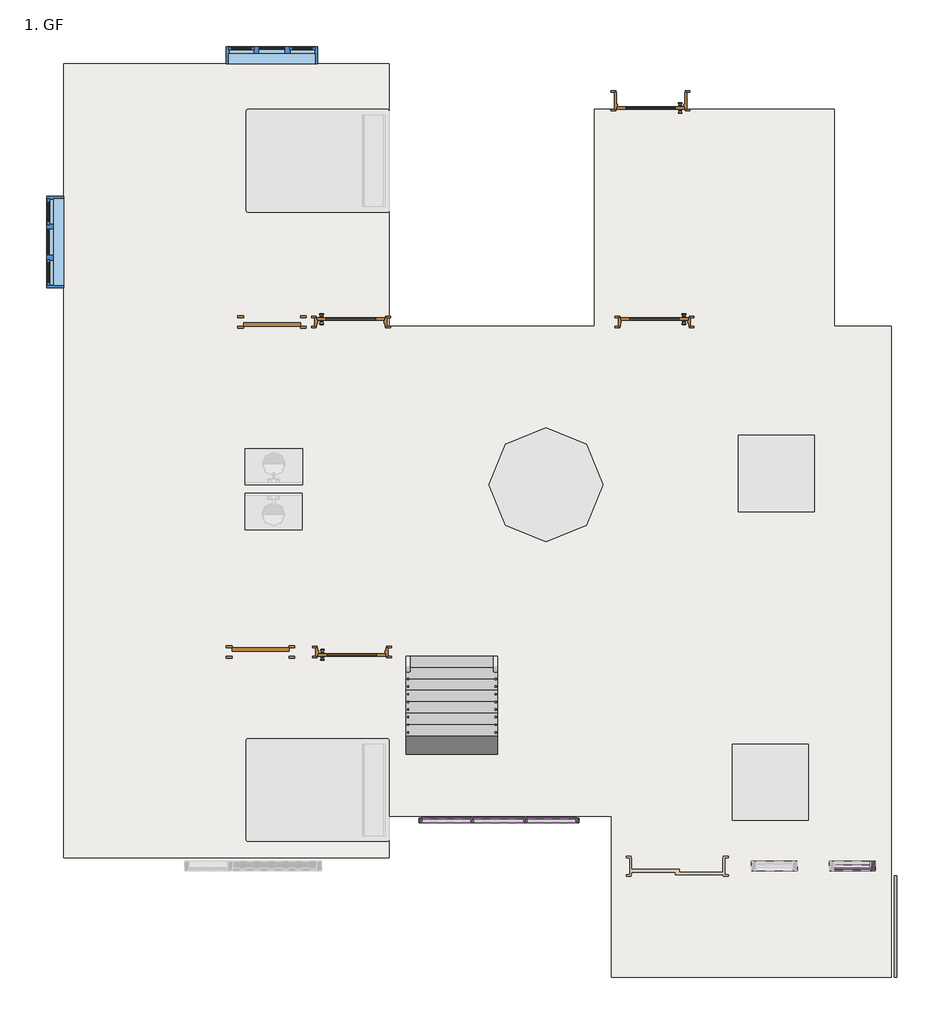
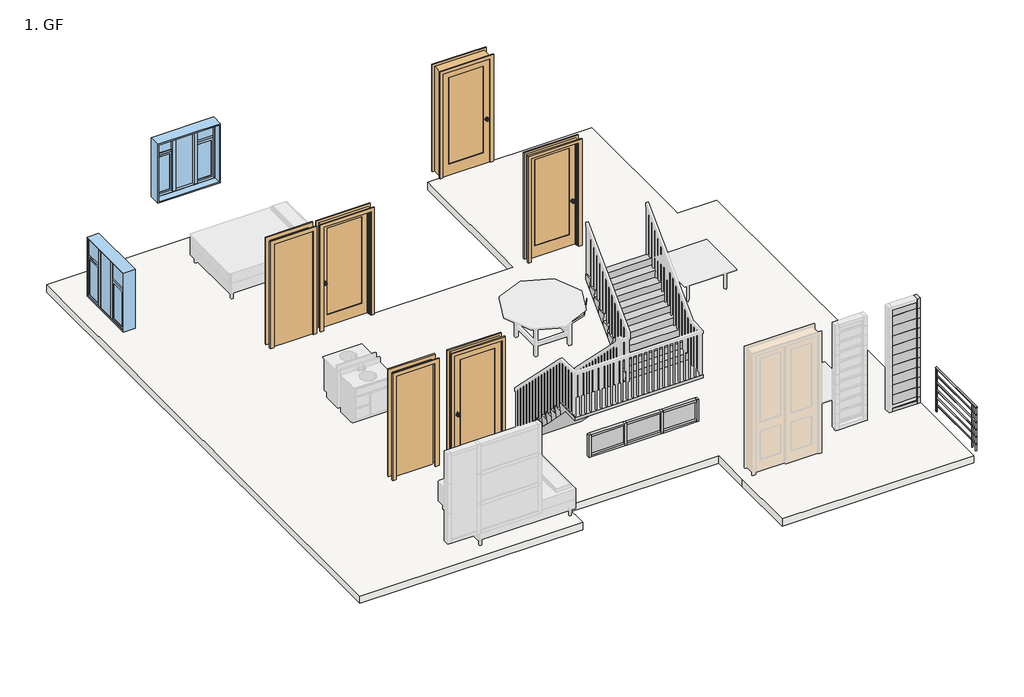
# One storey, part 2 of 3: 22 members, 13 plates, 6 doors, 2 windows, 1 railing, 1 slab, 1 stair flight.
"""IFC4 building model written with IfcOpenShell, lengths in millimetres."""

from ifc_helpers import new_model, si_unit, point, frame, frame_2d, origin, place, context, project, spatial, polyline, circle_curve, trimmed, segment, composite_curve, outline, extrude, faceted_brep, transform, mapped, element, save
from components import door_interior_single_1_panel_wood_4_x7_a3feeac7, door_interior_single_1_panel_wood_4_x7_3c6ab76a, door_interior_single_1_panel_wood_4_x7_3b97b8e7, door_214872d5, door_78caadf7, member_92f0adee, member_bf4473fa, member_7f78ed44, member_f6fe811f, member_86d06fe4, member_a8054089, member_a8e3eee7, system_panel_glazed_9eb8e914, system_panel_glazed_008e37cc, system_panel_glazed_f5251298, system_panel_glazed_d62326f9, window_casement_triple_side_transom_4_x4_fd24aed3

model = new_model("IFC4")

# Units and contexts
model_context = context("Model", 3, world=origin())
ifc_project = project(units=[si_unit("LENGTHUNIT", "METRE", prefix="MILLI")], contexts=[model_context])

# Site, building, storey
site = spatial("IfcSite", under=ifc_project)
building = spatial("IfcBuilding", under=site)
storey = spatial("IfcBuildingStorey", under=building, Name="1. GF", Elevation=609.6)

# Doors
placement = place(None, origin())
door_interior_single_1_panel_wood_4_x7_shape = door_interior_single_1_panel_wood_4_x7_a3feeac7(model_context)
element("IfcDoor", 1, ObjectType="Door-Interior-Single-1_Panel-Wood : 4'X7'", at=placement, inside=storey, context=model_context, shape_type="MappedRepresentation", body=[
    mapped(door_interior_single_1_panel_wood_4_x7_shape, transform((-3488.3749552, 2247.2410289, 609.6), x_axis=(1.0, 0.0, 0.0), y_axis=(0.0, 1.0, 0.0), z_axis=(0.0, 0.0, 1.0))),
])
element("IfcDoor", 2, ObjectType="Door-Interior-Single-1_Panel-Wood : 4'X7'", at=placement, inside=storey, context=model_context, shape_type="MappedRepresentation", body=[
    mapped(door_interior_single_1_panel_wood_4_x7_shape, transform((550.2250448, 6654.1410289, 609.6), x_axis=(-1.0, 0.0, 0.0), y_axis=(0.0, -1.0, 0.0), z_axis=(0.0, 0.0, 1.0))),
])
door_interior_single_1_panel_wood_4_x7_2_shape = door_interior_single_1_panel_wood_4_x7_3c6ab76a(model_context)
element("IfcDoor", 3, ObjectType="Door-Interior-Single-1_Panel-Wood : 4'X7'", at=placement, inside=storey, context=model_context, shape_type="MappedRepresentation", body=[
    mapped(door_interior_single_1_panel_wood_4_x7_2_shape, transform((-3501.0749552, 6654.1410289, 609.6), x_axis=(1.0, 0.0, 0.0), y_axis=(0.0, 1.0, 0.0), z_axis=(0.0, 0.0, 1.0))),
])
door_interior_single_1_panel_wood_4_x7_3_shape = door_interior_single_1_panel_wood_4_x7_3b97b8e7(model_context)
element("IfcDoor", 4, ObjectType="Door-Interior-Single-1_Panel-Wood : 4'X7'", at=placement, inside=storey, context=model_context, shape_type="MappedRepresentation", body=[
    mapped(door_interior_single_1_panel_wood_4_x7_3_shape, transform((499.4250448, 9600.5410289, 609.6), x_axis=(-1.0, 0.0, 0.0), y_axis=(0.0, -1.0, 0.0), z_axis=(0.0, 0.0, 1.0))),
])
door_shape = door_214872d5(model_context)
element("IfcDoor", 5, ObjectType="Single-Flush : 2'6\" X 7'", at=placement, inside=storey, context=model_context, shape_type="MappedRepresentation", body=[
    mapped(door_shape, transform((-4707.5749552, 2250.4160289, 609.6), x_axis=(1.0, 0.0, 0.0), y_axis=(0.0, 1.0, 0.0), z_axis=(0.0, 0.0, 1.0))),
])
door_2_shape = door_78caadf7(model_context)
element("IfcDoor", 6, ObjectType="Single-Flush : 2'6\" X 7'", at=placement, inside=storey, context=model_context, shape_type="MappedRepresentation", body=[
    mapped(door_2_shape, transform((-4555.1749552, 6650.9660289, 609.6), x_axis=(1.0, 0.0, 0.0), y_axis=(0.0, 1.0, 0.0), z_axis=(0.0, 0.0, 1.0))),
])

# Members
member_shape = member_92f0adee(model_context)
element("IfcMember", 7, ObjectType="Rectangular Mullion : 1.5\" x 2.5\" rectangular", at=placement, inside=storey, context=model_context, shape_type="MappedRepresentation", body=[
    mapped(member_shape, transform((-497.5249552, 2.5160289, 1981.2), x_axis=(0.0, 0.0, 1.0), y_axis=(0.0, -1.0, 0.0), z_axis=(1.0, 0.0, 0.0))),
])
element("IfcMember", 8, ObjectType="Rectangular Mullion : 1.5\" x 2.5\" rectangular", at=placement, inside=storey, context=model_context, shape_type="MappedRepresentation", body=[
    mapped(member_shape, transform((-1900.8749552, 2.5160289, 1981.2), x_axis=(0.0, 0.0, 1.0), y_axis=(0.0, -1.0, 0.0), z_axis=(1.0, 0.0, 0.0))),
])
element("IfcMember", 9, ObjectType="Rectangular Mullion : 1.5\" x 2.5\" rectangular", at=placement, inside=storey, context=model_context, shape_type="MappedRepresentation", body=[
    mapped(member_shape, transform((-2554.9249552, 2.5160289, 1524.0), x_axis=(0.0, 0.0, -1.0), y_axis=(0.0, -1.0, 0.0), z_axis=(-1.0, 0.0, 0.0))),
])
element("IfcMember", 10, ObjectType="Rectangular Mullion : 1.5\" x 2.5\" rectangular", at=placement, inside=storey, context=model_context, shape_type="MappedRepresentation", body=[
    mapped(member_shape, transform((-1151.5749552, 2.5160289, 1524.0), x_axis=(0.0, 0.0, -1.0), y_axis=(0.0, -1.0, 0.0), z_axis=(-1.0, 0.0, 0.0))),
])
member_2_shape = member_bf4473fa(model_context)
element("IfcMember", 11, ObjectType="Rectangular Mullion : 1.5\" x 2.5\" rectangular", at=placement, inside=storey, context=model_context, shape_type="MappedRepresentation", body=[
    mapped(member_2_shape, transform((-1881.8249552, 2.5160289, 1524.0), x_axis=(1.0, 0.0, 0.0), y_axis=(0.0, -1.0, 0.0), z_axis=(0.0, 0.0, -1.0))),
])
element("IfcMember", 12, ObjectType="Rectangular Mullion : 1.5\" x 2.5\" rectangular", at=placement, inside=storey, context=model_context, shape_type="MappedRepresentation", body=[
    mapped(member_2_shape, transform((-1170.6249552, 2.5160289, 1524.0), x_axis=(1.0, 0.0, 0.0), y_axis=(0.0, -1.0, 0.0), z_axis=(0.0, 0.0, -1.0))),
])
member_3_shape = member_7f78ed44(model_context)
element("IfcMember", 13, ObjectType="Rectangular Mullion : 1.5\" x 2.5\" rectangular", at=placement, inside=storey, context=model_context, shape_type="MappedRepresentation", body=[
    mapped(member_3_shape, transform((-1862.7749552, 2.5160289, 1524.0), x_axis=(0.0, 0.0, -1.0), y_axis=(0.0, -1.0, 0.0), z_axis=(-1.0, 0.0, 0.0))),
])
element("IfcMember", 14, ObjectType="Rectangular Mullion : 1.5\" x 2.5\" rectangular", at=placement, inside=storey, context=model_context, shape_type="MappedRepresentation", body=[
    mapped(member_3_shape, transform((-1189.6749552, 2.5160289, 1981.2), x_axis=(0.0, 0.0, 1.0), y_axis=(0.0, -1.0, 0.0), z_axis=(1.0, 0.0, 0.0))),
])
member_4_shape = member_f6fe811f(model_context)
element("IfcMember", 15, ObjectType="Rectangular Mullion : 1.5\" x 2.5\" rectangular", at=placement, inside=storey, context=model_context, shape_type="MappedRepresentation", body=[
    mapped(member_4_shape, transform((-2593.0249552, 2.5160289, 1981.2), x_axis=(-1.0, 0.0, 0.0), y_axis=(0.0, -1.0, 0.0), z_axis=(0.0, 0.0, 1.0))),
])
element("IfcMember", 16, ObjectType="Rectangular Mullion : 1.5\" x 2.5\" rectangular", at=placement, inside=storey, context=model_context, shape_type="MappedRepresentation", body=[
    mapped(member_4_shape, transform((-459.4249552, 2.5160289, 1524.0), x_axis=(1.0, 0.0, 0.0), y_axis=(0.0, -1.0, 0.0), z_axis=(0.0, 0.0, -1.0))),
])
member_5_shape = member_86d06fe4(model_context)
element("IfcMember", 17, ObjectType="Rectangular Mullion : 2.5\" x 5\" rectangular", at=placement, inside=storey, context=model_context, shape_type="MappedRepresentation", body=[
    mapped(member_5_shape, transform((3433.1250448, -607.0839711, 914.4), x_axis=(0.0, 0.0, -1.0), y_axis=(0.0, 1.0, 0.0), z_axis=(1.0, 0.0, 0.0))),
])
member_6_shape = member_a8054089(model_context)
element("IfcMember", 18, ObjectType="Rectangular Mullion : 2.5\" x 5\" rectangular", at=placement, inside=storey, context=model_context, shape_type="MappedRepresentation", body=[
    mapped(member_6_shape, transform((3496.6250448, -607.0839711, 3073.4), x_axis=(1.0, 0.0, 0.0), y_axis=(0.0, 1.0, 0.0), z_axis=(0.0, 0.0, 1.0))),
])
element("IfcMember", 19, ObjectType="Rectangular Mullion : 2.5\" x 5\" rectangular", at=placement, inside=storey, context=model_context, shape_type="MappedRepresentation", body=[
    mapped(member_6_shape, transform((3496.6250448, -607.0839711, 2870.2), x_axis=(1.0, 0.0, 0.0), y_axis=(0.0, 1.0, 0.0), z_axis=(0.0, 0.0, 1.0))),
])
element("IfcMember", 20, ObjectType="Rectangular Mullion : 2.5\" x 5\" rectangular", at=placement, inside=storey, context=model_context, shape_type="MappedRepresentation", body=[
    mapped(member_6_shape, transform((3496.6250448, -607.0839711, 2667.0), x_axis=(1.0, 0.0, 0.0), y_axis=(0.0, 1.0, 0.0), z_axis=(0.0, 0.0, 1.0))),
])
element("IfcMember", 21, ObjectType="Rectangular Mullion : 2.5\" x 5\" rectangular", at=placement, inside=storey, context=model_context, shape_type="MappedRepresentation", body=[
    mapped(member_6_shape, transform((3496.6250448, -607.0839711, 2463.8), x_axis=(1.0, 0.0, 0.0), y_axis=(0.0, 1.0, 0.0), z_axis=(0.0, 0.0, 1.0))),
])
element("IfcMember", 22, ObjectType="Rectangular Mullion : 2.5\" x 5\" rectangular", at=placement, inside=storey, context=model_context, shape_type="MappedRepresentation", body=[
    mapped(member_6_shape, transform((3496.6250448, -607.0839711, 2260.6), x_axis=(1.0, 0.0, 0.0), y_axis=(0.0, 1.0, 0.0), z_axis=(0.0, 0.0, 1.0))),
])
element("IfcMember", 23, ObjectType="Rectangular Mullion : 2.5\" x 5\" rectangular", at=placement, inside=storey, context=model_context, shape_type="MappedRepresentation", body=[
    mapped(member_6_shape, transform((3496.6250448, -607.0839711, 2057.4), x_axis=(1.0, 0.0, 0.0), y_axis=(0.0, 1.0, 0.0), z_axis=(0.0, 0.0, 1.0))),
])
element("IfcMember", 24, ObjectType="Rectangular Mullion : 2.5\" x 5\" rectangular", at=placement, inside=storey, context=model_context, shape_type="MappedRepresentation", body=[
    mapped(member_6_shape, transform((3496.6250448, -607.0839711, 1854.2), x_axis=(1.0, 0.0, 0.0), y_axis=(0.0, 1.0, 0.0), z_axis=(0.0, 0.0, 1.0))),
])
element("IfcMember", 25, ObjectType="Rectangular Mullion : 2.5\" x 5\" rectangular", at=placement, inside=storey, context=model_context, shape_type="MappedRepresentation", body=[
    mapped(member_6_shape, transform((3496.6250448, -607.0839711, 1651.0), x_axis=(1.0, 0.0, 0.0), y_axis=(0.0, 1.0, 0.0), z_axis=(0.0, 0.0, 1.0))),
])
element("IfcMember", 26, ObjectType="Rectangular Mullion : 2.5\" x 5\" rectangular", at=placement, inside=storey, context=model_context, shape_type="MappedRepresentation", body=[
    mapped(member_6_shape, transform((3496.6250448, -607.0839711, 1447.8), x_axis=(1.0, 0.0, 0.0), y_axis=(0.0, 1.0, 0.0), z_axis=(0.0, 0.0, 1.0))),
])
element("IfcMember", 27, ObjectType="Rectangular Mullion : 2.5\" x 5\" rectangular", at=placement, inside=storey, context=model_context, shape_type="MappedRepresentation", body=[
    mapped(member_6_shape, transform((3496.6250448, -607.0839711, 1244.6), x_axis=(1.0, 0.0, 0.0), y_axis=(0.0, 1.0, 0.0), z_axis=(0.0, 0.0, 1.0))),
])
member_7_shape = member_a8e3eee7(model_context)
element("IfcMember", 28, ObjectType="Rectangular Mullion : 2.5\" x 5\" rectangular", at=placement, inside=storey, context=model_context, shape_type="MappedRepresentation", body=[
    mapped(member_7_shape, transform((3496.6250448, -607.0839711, 1041.4), x_axis=(1.0, 0.0, 0.0), y_axis=(0.0, 1.0, 0.0), z_axis=(0.0, 0.0, 1.0))),
])

# Plates
system_panel_glazed_shape = system_panel_glazed_9eb8e914(model_context)
element("IfcPlate", 29, ObjectType="System Panel : Glazed", at=placement, inside=storey, context=model_context, shape_type="MappedRepresentation", body=[
    mapped(system_panel_glazed_shape, transform((3191.8250448, -607.0839711, 2667.0), x_axis=(-1.0, 0.0, 0.0), y_axis=(0.0, -1.0, 0.0), z_axis=(0.0, 0.0, 1.0))),
])
element("IfcPlate", 30, ObjectType="System Panel : Glazed", at=placement, inside=storey, context=model_context, shape_type="MappedRepresentation", body=[
    mapped(system_panel_glazed_shape, transform((3191.8250448, -607.0839711, 2463.8), x_axis=(-1.0, 0.0, 0.0), y_axis=(0.0, -1.0, 0.0), z_axis=(0.0, 0.0, 1.0))),
])
element("IfcPlate", 31, ObjectType="System Panel : Glazed", at=placement, inside=storey, context=model_context, shape_type="MappedRepresentation", body=[
    mapped(system_panel_glazed_shape, transform((3191.8250448, -607.0839711, 2260.6), x_axis=(-1.0, 0.0, 0.0), y_axis=(0.0, -1.0, 0.0), z_axis=(0.0, 0.0, 1.0))),
])
element("IfcPlate", 32, ObjectType="System Panel : Glazed", at=placement, inside=storey, context=model_context, shape_type="MappedRepresentation", body=[
    mapped(system_panel_glazed_shape, transform((3191.8250448, -607.0839711, 2057.4), x_axis=(-1.0, 0.0, 0.0), y_axis=(0.0, -1.0, 0.0), z_axis=(0.0, 0.0, 1.0))),
])
element("IfcPlate", 33, ObjectType="System Panel : Glazed", at=placement, inside=storey, context=model_context, shape_type="MappedRepresentation", body=[
    mapped(system_panel_glazed_shape, transform((3191.8250448, -607.0839711, 1854.2), x_axis=(-1.0, 0.0, 0.0), y_axis=(0.0, -1.0, 0.0), z_axis=(0.0, 0.0, 1.0))),
])
element("IfcPlate", 34, ObjectType="System Panel : Glazed", at=placement, inside=storey, context=model_context, shape_type="MappedRepresentation", body=[
    mapped(system_panel_glazed_shape, transform((3191.8250448, -607.0839711, 1651.0), x_axis=(-1.0, 0.0, 0.0), y_axis=(0.0, -1.0, 0.0), z_axis=(0.0, 0.0, 1.0))),
])
element("IfcPlate", 35, ObjectType="System Panel : Glazed", at=placement, inside=storey, context=model_context, shape_type="MappedRepresentation", body=[
    mapped(system_panel_glazed_shape, transform((3191.8250448, -607.0839711, 1447.8), x_axis=(-1.0, 0.0, 0.0), y_axis=(0.0, -1.0, 0.0), z_axis=(0.0, 0.0, 1.0))),
])
element("IfcPlate", 36, ObjectType="System Panel : Glazed", at=placement, inside=storey, context=model_context, shape_type="MappedRepresentation", body=[
    mapped(system_panel_glazed_shape, transform((3191.8250448, -607.0839711, 1244.6), x_axis=(-1.0, 0.0, 0.0), y_axis=(0.0, -1.0, 0.0), z_axis=(0.0, 0.0, 1.0))),
])
element("IfcPlate", 37, ObjectType="System Panel : Glazed", at=placement, inside=storey, context=model_context, shape_type="MappedRepresentation", body=[
    mapped(system_panel_glazed_shape, transform((3191.8250448, -607.0839711, 1041.4), x_axis=(-1.0, 0.0, 0.0), y_axis=(0.0, -1.0, 0.0), z_axis=(0.0, 0.0, 1.0))),
])
system_panel_glazed_2_shape = system_panel_glazed_008e37cc(model_context)
element("IfcPlate", 38, ObjectType="System Panel : Glazed", at=placement, inside=storey, context=model_context, shape_type="MappedRepresentation", body=[
    mapped(system_panel_glazed_2_shape, transform((3191.8250448, -607.0839711, 2870.2), x_axis=(-1.0, 0.0, 0.0), y_axis=(0.0, -1.0, 0.0), z_axis=(0.0, 0.0, 1.0))),
])
system_panel_glazed_3_shape = system_panel_glazed_f5251298(model_context)
element("IfcPlate", 39, ObjectType="System Panel : Glazed", at=placement, inside=storey, context=model_context, shape_type="MappedRepresentation", body=[
    mapped(system_panel_glazed_3_shape, transform((-2227.8999552, 2.5160289, 1562.1), x_axis=(1.0, 0.0, 0.0), y_axis=(0.0, 1.0, 0.0), z_axis=(0.0, 0.0, 1.0))),
])
element("IfcPlate", 40, ObjectType="System Panel : Glazed", at=placement, inside=storey, context=model_context, shape_type="MappedRepresentation", body=[
    mapped(system_panel_glazed_3_shape, transform((-824.5499552, 2.5160289, 1562.1), x_axis=(1.0, 0.0, 0.0), y_axis=(0.0, 1.0, 0.0), z_axis=(0.0, 0.0, 1.0))),
])
system_panel_glazed_4_shape = system_panel_glazed_d62326f9(model_context)
element("IfcPlate", 41, ObjectType="System Panel : Glazed", at=placement, inside=storey, context=model_context, shape_type="MappedRepresentation", body=[
    mapped(system_panel_glazed_4_shape, transform((-1526.2249552, 2.5160289, 1562.1), x_axis=(1.0, 0.0, 0.0), y_axis=(0.0, 1.0, 0.0), z_axis=(0.0, 0.0, 1.0))),
])

# Railing
element("IfcRailing", 42, ObjectType="Handrail - Pipe", at=placement, inside=storey, context=model_context, shape_type="SweptSolid", body=[
    extrude(outline(composite_curve([segment(trimmed(circle_curve(frame_2d((1579.959375, 3769.6750448)), 19.05), [point((1579.959375, 3750.6250448))], [point((1579.959375, 3788.7250448))], False, "CARTESIAN"), True, "CONTINUOUS"), segment(trimmed(circle_curve(frame_2d((1579.959375, 3769.6750448)), 19.05), [point((1579.959375, 3788.7250448))], [point((1579.959375, 3750.6250448))], False, "CARTESIAN"), True, "CONTINUOUS")], self_intersect=False)), frame((0.0, -2092.7839711, 0.0), z_axis=(0.0, 1.0, 0.0), x_axis=(0.0, 0.0, 1.0)), (0.0, 0.0, 1.0), 1358.7),
    extrude(outline(composite_curve([segment(trimmed(circle_curve(frame_2d((1433.909375, 3769.6750448)), 12.7), [point((1433.909375, 3782.3750448))], [point((1433.909375, 3756.9750448))], False, "CARTESIAN"), True, "CONTINUOUS"), segment(trimmed(circle_curve(frame_2d((1433.909375, 3769.6750448)), 12.7), [point((1433.909375, 3756.9750448))], [point((1433.909375, 3782.3750448))], False, "CARTESIAN"), True, "CONTINUOUS")], self_intersect=False)), frame((0.0, -2092.7839711, 0.0), z_axis=(0.0, 1.0, 0.0), x_axis=(0.0, 0.0, 1.0)), (0.0, 0.0, 1.0), 1358.7),
    extrude(outline(composite_curve([segment(trimmed(circle_curve(frame_2d((1281.509375, 3769.6750448)), 12.7), [point((1281.509375, 3782.3750448))], [point((1281.509375, 3756.9750448))], False, "CARTESIAN"), True, "CONTINUOUS"), segment(trimmed(circle_curve(frame_2d((1281.509375, 3769.6750448)), 12.7), [point((1281.509375, 3756.9750448))], [point((1281.509375, 3782.3750448))], False, "CARTESIAN"), True, "CONTINUOUS")], self_intersect=False)), frame((0.0, -2092.7839711, 0.0), z_axis=(0.0, 1.0, 0.0), x_axis=(0.0, 0.0, 1.0)), (0.0, 0.0, 1.0), 1358.7),
    extrude(outline(composite_curve([segment(trimmed(circle_curve(frame_2d((1129.109375, 3769.6750448)), 12.7), [point((1129.109375, 3782.3750448))], [point((1129.109375, 3756.9750448))], False, "CARTESIAN"), True, "CONTINUOUS"), segment(trimmed(circle_curve(frame_2d((1129.109375, 3769.6750448)), 12.7), [point((1129.109375, 3756.9750448))], [point((1129.109375, 3782.3750448))], False, "CARTESIAN"), True, "CONTINUOUS")], self_intersect=False)), frame((0.0, -2092.7839711, 0.0), z_axis=(0.0, 1.0, 0.0), x_axis=(0.0, 0.0, 1.0)), (0.0, 0.0, 1.0), 1358.7),
    extrude(outline(composite_curve([segment(trimmed(circle_curve(frame_2d((976.709375, 3769.6750448)), 12.7), [point((976.709375, 3782.3750448))], [point((976.709375, 3756.9750448))], False, "CARTESIAN"), True, "CONTINUOUS"), segment(trimmed(circle_curve(frame_2d((976.709375, 3769.6750448)), 12.7), [point((976.709375, 3756.9750448))], [point((976.709375, 3782.3750448))], False, "CARTESIAN"), True, "CONTINUOUS")], self_intersect=False)), frame((0.0, -2092.7839711, 0.0), z_axis=(0.0, 1.0, 0.0), x_axis=(0.0, 0.0, 1.0)), (0.0, 0.0, 1.0), 1358.7),
    extrude(outline(composite_curve([segment(trimmed(circle_curve(frame_2d((824.309375, 3769.6750448)), 12.7), [point((824.309375, 3782.3750448))], [point((824.309375, 3756.9750448))], False, "CARTESIAN"), True, "CONTINUOUS"), segment(trimmed(circle_curve(frame_2d((824.309375, 3769.6750448)), 12.7), [point((824.309375, 3756.9750448))], [point((824.309375, 3782.3750448))], False, "CARTESIAN"), True, "CONTINUOUS")], self_intersect=False)), frame((0.0, -2092.7839711, 0.0), z_axis=(0.0, 1.0, 0.0), x_axis=(0.0, 0.0, 1.0)), (0.0, 0.0, 1.0), 1358.7),
    extrude(outline(composite_curve([segment(trimmed(circle_curve(frame_2d((3769.6750448, -1953.2839711)), 12.7), [point((3782.3750448, -1953.2839711))], [point((3756.9750448, -1953.2839711))], False, "CARTESIAN"), True, "CONTINUOUS"), segment(trimmed(circle_curve(frame_2d((3769.6750448, -1953.2839711)), 12.7), [point((3756.9750448, -1953.2839711))], [point((3782.3750448, -1953.2839711))], False, "CARTESIAN"), True, "CONTINUOUS")], self_intersect=False)), frame((0.0, 0.0, 684.609375), z_axis=(0.0, 0.0, 1.0), x_axis=(1.0, 0.0, 0.0)), (0.0, 0.0, 1.0), 876.3),
    extrude(outline(composite_curve([segment(trimmed(circle_curve(frame_2d((3769.6750448, -2080.0839711)), 12.7), [point((3782.3750448, -2080.0839711))], [point((3756.9750448, -2080.0839711))], False, "CARTESIAN"), True, "CONTINUOUS"), segment(trimmed(circle_curve(frame_2d((3769.6750448, -2080.0839711)), 12.7), [point((3756.9750448, -2080.0839711))], [point((3782.3750448, -2080.0839711))], False, "CARTESIAN"), True, "CONTINUOUS")], self_intersect=False)), frame((0.0, 0.0, 684.609375), z_axis=(0.0, 0.0, 1.0), x_axis=(1.0, 0.0, 0.0)), (0.0, 0.0, 1.0), 876.3),
    extrude(outline(composite_curve([segment(trimmed(circle_curve(frame_2d((3769.6750448, -746.7839711)), 12.7), [point((3782.3750448, -746.7839711))], [point((3756.9750448, -746.7839711))], False, "CARTESIAN"), True, "CONTINUOUS"), segment(trimmed(circle_curve(frame_2d((3769.6750448, -746.7839711)), 12.7), [point((3756.9750448, -746.7839711))], [point((3782.3750448, -746.7839711))], False, "CARTESIAN"), True, "CONTINUOUS")], self_intersect=False)), frame((0.0, 0.0, 684.609375), z_axis=(0.0, 0.0, 1.0), x_axis=(1.0, 0.0, 0.0)), (0.0, 0.0, 1.0), 876.3),
])

# Slab
element("IfcSlab", 43, ObjectType="6\" FLOOR", at=placement, inside=storey, context=model_context, shape_type="SweptSolid", body=[
    extrude(outline(polyline([(-2993.0749552, 10099.0160289), (-2993.0749552, 6593.8160289), (-249.8749552, 6593.8160289), (-249.8749552, 9489.4160289), (2950.5250448, 9489.4160289), (2950.5250448, 6708.1160289), (2950.5250448, 6593.8160289), (3712.5250448, 6593.8160289), (3712.5250448, -492.7839711), (3712.5250448, -2092.7839711), (-21.2749552, -2092.7839711), (-21.2749552, -728.4733894), (-21.2749552, 59.6660289), (-2993.0749552, 59.6660289), (-2993.0749552, -492.7839711), (-7336.4749552, -492.7839711), (-7336.4749552, 10099.0160289), (-2993.0749552, 10099.0160289)])), frame((0.0, 0.0, 457.2), z_axis=(0.0, 0.0, 1.0), x_axis=(1.0, 0.0, 0.0)), (0.0, 0.0, 1.0), 152.4),
])

# Stair flight
element("IfcStairFlight", 44, ObjectType="3/4\" Nosing", at=placement, inside=storey, context=model_context, shape_type="Brep", body=[
    faceted_brep([(-2764.4749552, 2193.2660289, 762.0), (-1545.2749552, 2193.2660289, 762.0), (-1545.2749552, 2174.2160289, 609.6), (-2764.4749552, 2174.2160289, 609.6), (-2764.4749552, 2021.8160289, 762.0), (-1545.2749552, 2021.8160289, 762.0), (-1545.2749552, 2021.8160289, 672.1974388), (-1545.2749552, 2084.4134676, 609.6), (-2764.4749552, 2084.4134676, 609.6), (-2764.4749552, 2021.8160289, 672.1974388), (-1545.2749552, 2040.8660289, 914.4), (-2764.4749552, 2040.8660289, 914.4), (-2764.4749552, 1869.4160289, 914.4), (-1545.2749552, 1869.4160289, 914.4), (-1545.2749552, 1869.4160289, 824.5974388), (-2764.4749552, 1869.4160289, 824.5974388), (-1545.2749552, 1888.4660289, 1066.8), (-2764.4749552, 1888.4660289, 1066.8), (-2764.4749552, 1717.0160289, 1066.8), (-1545.2749552, 1717.0160289, 1066.8), (-1545.2749552, 1717.0160289, 976.9974388), (-2764.4749552, 1717.0160289, 976.9974388), (-1545.2749552, 1736.0660289, 1219.2), (-2764.4749552, 1736.0660289, 1219.2), (-2764.4749552, 1564.6160289, 1219.2), (-1545.2749552, 1564.6160289, 1219.2), (-1545.2749552, 1564.6160289, 1129.3974388), (-2764.4749552, 1564.6160289, 1129.3974388), (-1545.2749552, 1583.6660289, 1371.6), (-2764.4749552, 1583.6660289, 1371.6), (-2764.4749552, 1412.2160289, 1371.6), (-1545.2749552, 1412.2160289, 1371.6), (-1545.2749552, 1412.2160289, 1281.7974388), (-2764.4749552, 1412.2160289, 1281.7974388), (-1545.2749552, 1431.2660289, 1524.0), (-2764.4749552, 1431.2660289, 1524.0), (-2764.4749552, 1259.8160289, 1524.0), (-1545.2749552, 1259.8160289, 1524.0), (-1545.2749552, 1259.8160289, 1434.1974388), (-2764.4749552, 1259.8160289, 1434.1974388), (-1545.2749552, 1278.8660289, 1676.4), (-2764.4749552, 1278.8660289, 1676.4), (-2764.4749552, 1107.4160289, 1676.4), (-1545.2749552, 1107.4160289, 1676.4), (-1545.2749552, 1107.4160289, 1586.5974388), (-2764.4749552, 1107.4160289, 1586.5974388), (-1545.2749552, 1126.4660289, 1828.8), (-2764.4749552, 1126.4660289, 1828.8), (-2764.4749552, 955.0160289, 1828.8), (-1545.2749552, 955.0160289, 1828.8), (-1545.2749552, 955.0160289, 1738.9974388), (-2764.4749552, 955.0160289, 1738.9974388), (-1545.2749552, 974.0660289, 1981.2), (-2764.4749552, 974.0660289, 1981.2), (-2764.4749552, 802.6160289, 1981.2), (-1545.2749552, 802.6160289, 1981.2), (-1545.2749552, 802.6160289, 1891.3974388), (-2764.4749552, 802.6160289, 1891.3974388), (-1545.2749552, 650.2160289, 2133.6), (-1545.2749552, 821.6660289, 2133.6), (-2764.4749552, 821.6660289, 2133.6), (-2764.4749552, 650.2160289, 2133.6), (-1545.2749552, 661.3285289, 2222.5), (-1545.2749552, 471.5134676, 2222.5), (-2764.4749552, 650.2160289, 2043.7974388), (-1469.0749552, 688.3160289, 2286.0), (-1469.0749552, 669.2660289, 2286.0), (-1545.2749552, 669.2660289, 2286.0), (-2764.4749552, 669.2660289, 2286.0), (-2764.4749552, 471.5134676, 2286.0), (-2764.4749552, 173.9660289, 2286.0), (-249.8749552, 173.9660289, 2286.0), (-249.8749552, 688.3160289, 2286.0), (-1469.0749552, 688.3160289, 2222.5), (-1469.0749552, 669.2660289, 2222.5), (-1545.2749552, 669.2660289, 2222.5), (-2764.4749552, 471.5134676, 2222.5), (-2764.4749552, 173.9660289, 2222.5), (-249.8749552, 173.9660289, 2222.5), (-249.8749552, 688.3160289, 2222.5), (-1469.0749552, 669.2660289, 2438.4), (-249.8749552, 669.2660289, 2438.4), (-249.8749552, 714.6185901, 2438.4), (-249.8749552, 840.7160289, 2438.4), (-1469.0749552, 840.7160289, 2438.4), (-1469.0749552, 714.6185901, 2438.4), (-1469.0749552, 840.7160289, 2348.5974388), (-1469.0749552, 714.6185901, 2222.5), (-249.8749552, 714.6185901, 2222.5), (-249.8749552, 840.7160289, 2348.5974388), (-1469.0749552, 821.6660289, 2590.8), (-249.8749552, 821.6660289, 2590.8), (-249.8749552, 993.1160289, 2590.8), (-1469.0749552, 993.1160289, 2590.8), (-1469.0749552, 993.1160289, 2500.9974388), (-249.8749552, 993.1160289, 2500.9974388), (-1469.0749552, 974.0660289, 2743.2), (-249.8749552, 974.0660289, 2743.2), (-249.8749552, 1145.5160289, 2743.2), (-1469.0749552, 1145.5160289, 2743.2), (-1469.0749552, 1145.5160289, 2653.3974388), (-249.8749552, 1145.5160289, 2653.3974388), (-1469.0749552, 1126.4660289, 2895.6), (-249.8749552, 1126.4660289, 2895.6), (-249.8749552, 1297.9160289, 2895.6), (-1469.0749552, 1297.9160289, 2895.6), (-1469.0749552, 1297.9160289, 2805.7974388), (-249.8749552, 1297.9160289, 2805.7974388), (-1469.0749552, 1278.8660289, 3048.0), (-249.8749552, 1278.8660289, 3048.0), (-249.8749552, 1450.3160289, 3048.0), (-1469.0749552, 1450.3160289, 3048.0), (-1469.0749552, 1450.3160289, 2958.1974388), (-249.8749552, 1450.3160289, 2958.1974388), (-1469.0749552, 1431.2660289, 3200.4), (-249.8749552, 1431.2660289, 3200.4), (-249.8749552, 1602.7160289, 3200.4), (-1469.0749552, 1602.7160289, 3200.4), (-1469.0749552, 1602.7160289, 3110.5974388), (-249.8749552, 1602.7160289, 3110.5974388), (-1469.0749552, 1583.6660289, 3352.8), (-249.8749552, 1583.6660289, 3352.8), (-249.8749552, 1755.1160289, 3352.8), (-1469.0749552, 1755.1160289, 3352.8), (-1469.0749552, 1755.1160289, 3262.9974388), (-249.8749552, 1755.1160289, 3262.9974388), (-1469.0749552, 1736.0660289, 3505.2), (-249.8749552, 1736.0660289, 3505.2), (-249.8749552, 1907.5160289, 3505.2), (-1469.0749552, 1907.5160289, 3505.2), (-1469.0749552, 1907.5160289, 3415.3974388), (-249.8749552, 1907.5160289, 3415.3974388), (-1469.0749552, 1888.4660289, 3657.6), (-249.8749552, 1888.4660289, 3657.6), (-249.8749552, 2040.8660289, 3657.6), (-1469.0749552, 2040.8660289, 3657.6), (-1469.0749552, 2040.8660289, 3548.7474388), (-249.8749552, 2040.8660289, 3548.7474388)], [[[0, 1, 2, 3]], [[1, 0, 4, 5]], [[1, 5, 6, 7, 2]], [[4, 0, 3, 8, 9]], [[10, 11, 12, 13]], [[10, 13, 14, 6, 5]], [[12, 11, 4, 9, 15]], [[5, 4, 11, 10]], [[16, 17, 18, 19]], [[16, 19, 20, 14, 13]], [[18, 17, 12, 15, 21]], [[13, 12, 17, 16]], [[22, 23, 24, 25]], [[22, 25, 26, 20, 19]], [[24, 23, 18, 21, 27]], [[19, 18, 23, 22]], [[28, 29, 30, 31]], [[28, 31, 32, 26, 25]], [[30, 29, 24, 27, 33]], [[25, 24, 29, 28]], [[34, 35, 36, 37]], [[34, 37, 38, 32, 31]], [[36, 35, 30, 33, 39]], [[31, 30, 35, 34]], [[40, 41, 42, 43]], [[40, 43, 44, 38, 37]], [[42, 41, 36, 39, 45]], [[37, 36, 41, 40]], [[46, 47, 48, 49]], [[46, 49, 50, 44, 43]], [[48, 47, 42, 45, 51]], [[43, 42, 47, 46]], [[52, 53, 54, 55]], [[52, 55, 56, 50, 49]], [[54, 53, 48, 51, 57]], [[49, 48, 53, 52]], [[58, 59, 60, 61]], [[58, 62, 63, 56, 55, 59]], [[61, 60, 54, 57, 64]], [[55, 54, 60, 59]], [[65, 66, 67, 68, 69, 70, 71, 72]], [[66, 65, 73, 74]], [[67, 66, 74, 75]], [[62, 67, 75]], [[68, 61, 64, 76, 77, 70, 69]], [[71, 70, 77, 78]], [[72, 71, 78, 79]], [[58, 61, 68, 67, 62]], [[80, 81, 82, 83, 84, 85]], [[65, 80, 85, 84, 86, 87, 73]], [[81, 72, 79, 88, 89, 83, 82]], [[65, 72, 81, 80]], [[90, 91, 92, 93]], [[90, 93, 94, 86, 84]], [[92, 91, 83, 89, 95]], [[84, 83, 91, 90]], [[96, 97, 98, 99]], [[96, 99, 100, 94, 93]], [[98, 97, 92, 95, 101]], [[93, 92, 97, 96]], [[102, 103, 104, 105]], [[102, 105, 106, 100, 99]], [[104, 103, 98, 101, 107]], [[99, 98, 103, 102]], [[108, 109, 110, 111]], [[108, 111, 112, 106, 105]], [[110, 109, 104, 107, 113]], [[105, 104, 109, 108]], [[114, 115, 116, 117]], [[114, 117, 118, 112, 111]], [[116, 115, 110, 113, 119]], [[111, 110, 115, 114]], [[120, 121, 122, 123]], [[120, 123, 124, 118, 117]], [[122, 121, 116, 119, 125]], [[117, 116, 121, 120]], [[126, 127, 128, 129]], [[126, 129, 130, 124, 123]], [[128, 127, 122, 125, 131]], [[123, 122, 127, 126]], [[132, 133, 134, 135]], [[132, 135, 136, 130, 129]], [[134, 133, 128, 131, 137]], [[135, 134, 137, 136]], [[129, 128, 133, 132]], [[3, 2, 7, 8]], [[56, 63, 76, 64, 57, 51, 45, 39, 33, 27, 21, 15, 9, 8, 7, 6, 14, 20, 26, 32, 38, 44, 50]], [[76, 63, 62, 75, 74, 73, 87, 88, 79, 78, 77]], [[88, 87, 86, 94, 100, 106, 112, 118, 124, 130, 136, 137, 131, 125, 119, 113, 107, 101, 95, 89]]]),
])

# Windows
window_casement_triple_side_transom_4_x4_shape = window_casement_triple_side_transom_4_x4_fd24aed3(model_context)
element("IfcWindow", 45, ObjectType="Window-Casement-Triple-Side-Transom : 4'x4'", at=placement, inside=storey, context=model_context, shape_type="MappedRepresentation", body=[
    mapped(window_casement_triple_side_transom_4_x4_shape, transform((-4555.1749552, 10213.3160289, 609.6), x_axis=(1.0, 0.0, 0.0), y_axis=(0.0, 1.0, 0.0), z_axis=(0.0, 0.0, 1.0))),
])
element("IfcWindow", 46, ObjectType="Window-Casement-Triple-Side-Transom : 4'x4'", at=placement, inside=storey, context=model_context, shape_type="MappedRepresentation", body=[
    mapped(window_casement_triple_side_transom_4_x4_shape, transform((-7450.7749552, 7717.7660289, 609.6), x_axis=(0.0, 1.0, 0.0), y_axis=(-1.0, 0.0, 0.0), z_axis=(0.0, 0.0, 1.0))),
])

save(model, "model.ifc")

# Revit data of these elements
# Type "Door-Interior-Single-1_Panel-Wood : 4'X7'"
#   Type Mark = "9"
#   Assembly Code = "C1020300"
#   Analytic Construction = "Wooden"
#   Top Rail = 0' - 4 11/16"
#   Thickness = 0' - 1 3/8"
#   Thermal Resistance (R) = 2.5876 (h·ft²·°F)/BTU
#   Swing Angle [instance default] = 90.00°
#   Stiles = 0' - 4 3/4"
#   Rough Width = 3' - 2"
#   Rough Height = 7' - 1"
#   Height = 7' - 0"
#   Width = 3' - 0"
#   Heat Transfer Coefficient (U) = 0.3865 BTU/(h·ft²·°F)
#   Bottom Rail = 0' - 9 1/8"
#   Trim Material = Cherry
#   Panel Material = Cherry
#   Frame Material = Cherry
#   Door Handle Material = Aluminum
#   Visual Light Transmittance = 0
#   Solar Heat Gain Coefficient = 0
#   Wall Closure = (empty or 0)
#   Function = (empty or 0)
# Type "Single-Flush : 2'6\" X 7'"
#   Type Mark = "14"
#   Construction Type Id = "MDOOR"
#   Assembly Code = "C1020"
#   Analytic Construction = "Metal"
#   Thickness = 0' - 2"
#   Heat Transfer Coefficient (U) = 0.651978 BTU/(h·ft²·°F)
#   Height = 7' - 0"
#   Trim Projection Ext = 0' - 1"
#   Trim Projection Int = 0' - 1"
#   Trim Width = 0' - 3"
#   Width = 2' - 6"
#   Define Thermal Properties by = 1
#   Door Material = Door - Panel
#   Frame Material = Door - Frame
#   Visual Light Transmittance = 0
#   Solar Heat Gain Coefficient = 0
#   Function = (empty or 0)
#   Wall Closure = (empty or 0)
# Type "Rectangular Mullion : 1.5\" x 2.5\" rectangular"
#   built-in parameter 1007304 = 0.208333 (stored number, unit not read)
#   built-in parameter 1007301 = 0.0625 (stored number, unit not read)
#   built-in parameter 1007300 = 0.0625 (stored number, unit not read)
# Type "Rectangular Mullion : 2.5\" x 5\" rectangular"
#   built-in parameter 1007304 = 0.416667 (stored number, unit not read)
#   built-in parameter 1007301 = 0.104167 (stored number, unit not read)
#   built-in parameter 1007300 = 0.104167 (stored number, unit not read)
# Type "System Panel : Glazed"
#   Construction Type Id = "GSP4R"
#   Analytic Construction = "1/8 in Pilkington single glazing"
#   Visual Light Transmittance = 0.9
#   Solar Heat Gain Coefficient = 0.86
#   Heat Transfer Coefficient (U) = 1.18115 BTU/(h·ft²·°F)
#   Define Thermal Properties by = 1
# Type "Handrail - Pipe"
#   Assembly Code = "C2010400"
#   built-in parameter 1008612 = 0.0416667 (stored number, unit not read)
#   built-in parameter 1008611 = 0.0833333 (stored number, unit not read)
#   built-in parameter 1008609 = 4 (stored number, unit not read)
#   built-in parameter 1008604 = 0.166667 (stored number, unit not read)
#   built-in parameter 1008603 = 0.166667 (stored number, unit not read)
#   Railing Height = 3' - 0"
#   built-in parameter 1008630 = 2
#   built-in parameter 1008610 = 1
#   built-in parameter 1008605 = 1
#   built-in parameter 1008618 = Baluster - Round : 1"
# Type "6\" FLOOR"
#   Assembly Code = "B1010"
#   Function = 0
#   Layers, outside or top first: 0' - 6" "Gypsum Wall Board" (function 1)
# Type "Window-Casement-Triple-Side-Transom : 4'x4'"
#   Type Mark = "27"
#   Fire Rating = "0.5h"
#   Assembly Code = "B2020100"
#   Analytic Construction = "Double glazing - domestic"
#   Window Width = 1' - 4"
#   Window Inset [instance default] = 0' - 0 5/8"
#   Wall Thickness [instance default] = 0' - 6"
#   Visual Light Transmittance = 0.81
#   Transom Height Ratio = 0.3
#   Thermal Resistance (R) = 1.8146 (h·ft²·°F)/BTU
#   Solar Heat Gain Coefficient = 0.76
#   Rough Width = 4' - 0 1/2"
#   Rough Height = 4' - 0 1/2"
#   Open Window Height = 2' - 9.6"
#   Heat Transfer Coefficient (U) = 0.5511 BTU/(h·ft²·°F)
#   Height = 4' - 0"
#   Transom Height = 1' - 2.4"
#   Frame Gap 3 [instance default] = 0' - 1 83/128"
#   Frame Gap 2 [instance default] = 0' - 0 5/8"
#   Frame Gap 1 = 0' - 1 51/128"
#   Default Sill Height = 3' - 0"
#   Width = 4' - 0"
#   Frame Material = Metal - Aluminum
#   Glass Panel Material = Glass
#   Wall Closure = (empty or 0)
# Elements 1, 2, 3, 4 (IfcDoor, "Door-Interior-Single-1_Panel-Wood : 4'X7'")
#   Swing Angle = 90.00°
#   Phase Created = New Construction
#   Materials on its faces: "Cherry", "Aluminum"
# Elements 5, 6 (IfcDoor, "Single-Flush : 2'6\" X 7'")
#   Phase Created = New Construction
#   Materials on its faces: "Door - Frame", "Door - Panel"
# Elements 7, 8, 9, 10, 11, 12, 13, 14, 15, 16 (IfcMember, "Rectangular Mullion : 1.5\" x 2.5\" rectangular")
#   Phase Created = New Construction
#   Materials on its faces: "Leather - Black"
# Elements 17, 18, 19, 20, 21, 22, 23, 24, 25, 26, 27, 28 (IfcMember, "Rectangular Mullion : 2.5\" x 5\" rectangular")
#   Phase Created = New Construction
#   Materials on its faces: "Door - Frame"
# Elements 29, 30, 31, 32, 33, 34, 35, 36, 37, 38, 39, 40, 41 (IfcPlate, "System Panel : Glazed")
#   Phase Created = New Construction
#   Materials on its faces: "Glass"
# Element 42 (IfcRailing, "Handrail - Pipe")
#   built-in parameter 1008621 = 0.246094 (stored number, unit not read)
#   Phase Created = New Construction
# Element 43 (IfcSlab, "6\" FLOOR")
#   Height Offset From Level = 0' - 0"
#   Phase Created = New Construction
#   Materials on its faces: "Gypsum Wall Board"
# Element 44 (IfcStairFlight, "3/4\" Nosing")
#   Phase Created = New Construction
#   Materials on its faces: "Concrete, Cast-in-Place gray"
# Element 45 (IfcWindow, "Window-Casement-Triple-Side-Transom : 4'x4'")
#   Mark = "2"
#   Window Inset = 0' - 0 5/8"
#   Frame Gap 3 = 0' - 1 83/128"
#   Frame Gap 2 = 0' - 0 5/8"
#   Phase Created = New Construction
#   Materials on its faces: "Metal - Aluminum", "Glass"
# Element 46 (IfcWindow, "Window-Casement-Triple-Side-Transom : 4'x4'")
#   Mark = "3"
#   Window Inset = 0' - 0 5/8"
#   Frame Gap 3 = 0' - 1 83/128"
#   Frame Gap 2 = 0' - 0 5/8"
#   Phase Created = New Construction
#   Materials on its faces: "Metal - Aluminum", "Glass"
# Materials
#   "Cherry": class "Wood", colour RGB 226 177 128, transparency 0, Description = "Prunus Serotina", Cost = 0
#   "Aluminum": class "Metal", colour RGB 247 247 247, transparency 0, Description = "Aluminum 6061", Cost = 0
#   "Door - Panel": class "Wood", colour RGB 210 159 95, transparency 0, Cost = 0
#   "Door - Frame": colour RGB 118 70 51, transparency 0, Cost = 0
#   "Gypsum Wall Board": class "Generic", colour RGB 228 228 228, transparency 0, Description = "Gypsum Wall Board", Cost = 0
#   "Metal - Aluminum": class "Metal", colour RGB 247 247 247, transparency 0
#   "Glass": class "Glass", colour RGB 0 128 192, transparency 0.75, Description = "Soda Lime Glass", Cost = 0
#   "Leather - Black": class "Generic", colour RGB 40 40 40, transparency 0, Cost = 0
#   "Concrete, Cast-in-Place gray": class "Concrete", colour RGB 192 192 192, transparency 0, Description = "Cast-in-place concrete", Cost = 0
